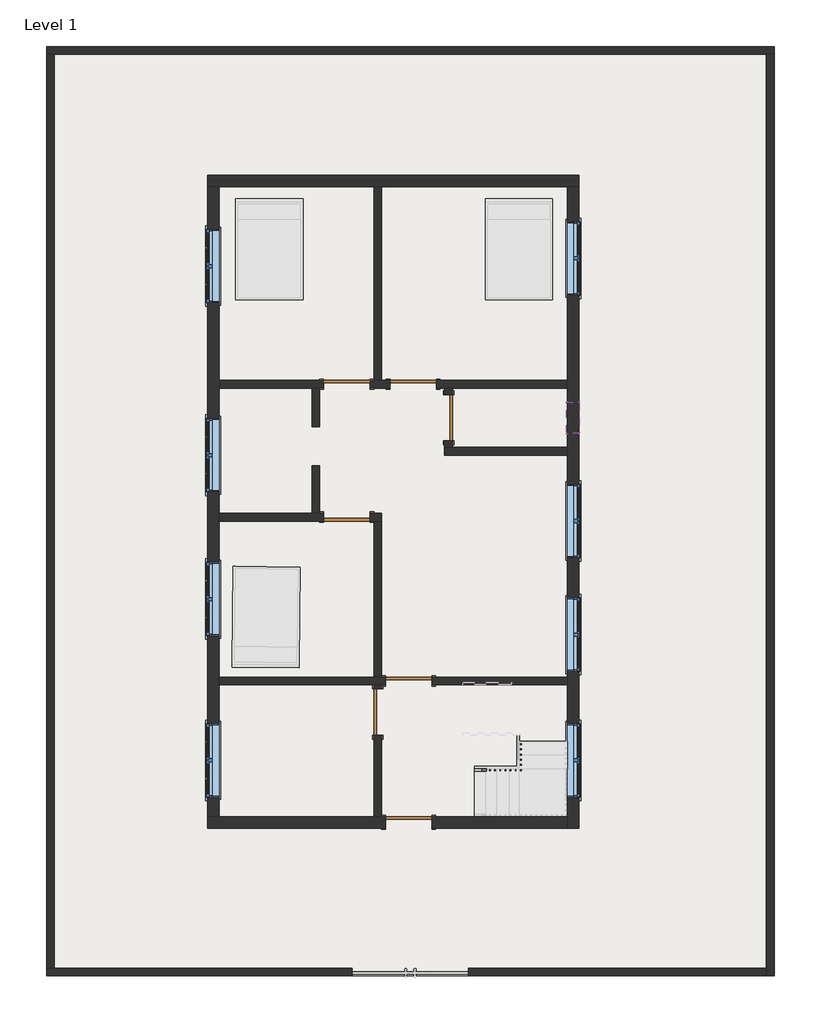
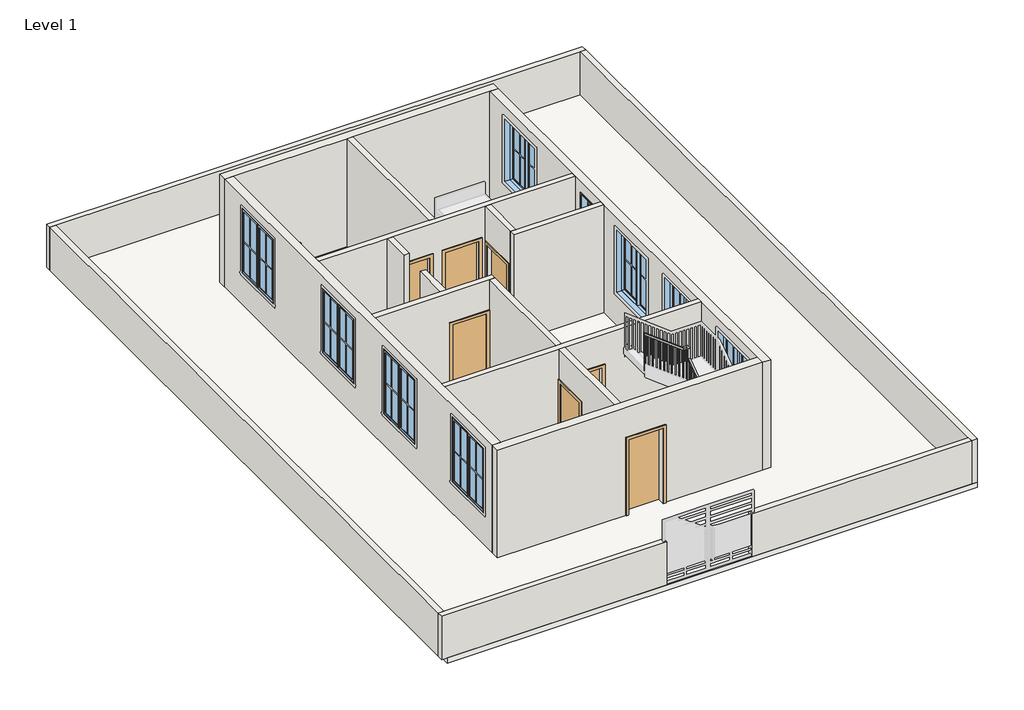
# One storey, part 1 of 2: 19 walls, 9 windows, 7 doors, 1 railing, 1 slab.
"""IFC4 building model written with IfcOpenShell, lengths in millimetres."""

from ifc_helpers import new_model, si_unit, frame, origin, origin_with_axes, place, context, project, spatial, polyline, outline, extrude, faceted_brep, transform, mapped, element, save
from components import door_2b0b55a0, door_686f89d2, door_16372e1c, door_a90ba1ad, window_9ac97e1a, window_f2d8fef0

model = new_model("IFC4")

# Units and contexts
model_context = context("Model", 3, world=origin())
ifc_project = project(units=[si_unit("LENGTHUNIT", "METRE", prefix="MILLI")], contexts=[model_context])

# Site, building, storey
site = spatial("IfcSite", under=ifc_project)
building = spatial("IfcBuilding", under=site)
storey = spatial("IfcBuildingStorey", under=building, Name="Level 1", Elevation=0.0)

# Doors
placement = place(None, origin())
door_shape = door_2b0b55a0(model_context)
element("IfcDoor", 1, ObjectType="Single-Flush : 36\" x 80\"", at=placement, inside=storey, context=model_context, shape_type="MappedRepresentation", body=[
    mapped(door_shape, transform((-163.235885, 1707.4649429, 0.0), x_axis=(0.0, 1.0, 0.0), y_axis=(-1.0, 0.0, 0.0), z_axis=(0.0, 0.0, 1.0))),
])
door_2_shape = door_686f89d2(model_context)
element("IfcDoor", 2, ObjectType="Single-Flush : 36\" x 84\"", at=placement, inside=storey, context=model_context, shape_type="MappedRepresentation", body=[
    mapped(door_2_shape, transform((-861.735885, 2367.8649429, 0.0), x_axis=(-1.0, 0.0, 0.0), y_axis=(0.0, -1.0, 0.0), z_axis=(0.0, 0.0, 1.0))),
])
element("IfcDoor", 3, ObjectType="Single-Flush : 36\" x 84\"", at=placement, inside=storey, context=model_context, shape_type="MappedRepresentation", body=[
    mapped(door_2_shape, transform((-2169.835885, -248.3350571, 0.0), x_axis=(1.0, 0.0, 0.0), y_axis=(0.0, 1.0, 0.0), z_axis=(0.0, 0.0, 1.0))),
])
element("IfcDoor", 4, ObjectType="Single-Flush : 36\" x 84\"", at=placement, inside=storey, context=model_context, shape_type="MappedRepresentation", body=[
    mapped(door_2_shape, transform((-950.635885, -3474.1350571, 0.0), x_axis=(-1.0, 0.0, 0.0), y_axis=(0.0, -1.0, 0.0), z_axis=(0.0, 0.0, 1.0))),
])
door_3_shape = door_16372e1c(model_context)
element("IfcDoor", 5, ObjectType="Single-Flush : 36\" x 84\"", at=placement, inside=storey, context=model_context, shape_type="MappedRepresentation", body=[
    mapped(door_3_shape, transform((-2169.835885, 2367.8649429, 0.0), x_axis=(1.0, 0.0, 0.0), y_axis=(0.0, 1.0, 0.0), z_axis=(0.0, 0.0, 1.0))),
])
element("IfcDoor", 6, ObjectType="Single-Flush : 36\" x 84\"", at=placement, inside=storey, context=model_context, shape_type="MappedRepresentation", body=[
    mapped(door_3_shape, transform((-1560.235885, -4083.7350571, 0.0), x_axis=(0.0, 1.0, 0.0), y_axis=(-1.0, 0.0, 0.0), z_axis=(0.0, 0.0, 1.0))),
])
door_4_shape = door_a90ba1ad(model_context)
element("IfcDoor", 7, ObjectType="Single-Flush : 36\" x 84\"", at=placement, inside=storey, context=model_context, shape_type="MappedRepresentation", body=[
    mapped(door_4_shape, transform((-950.635885, -6255.4350571, 0.0), x_axis=(-1.0, 0.0, 0.0), y_axis=(0.0, -1.0, 0.0), z_axis=(0.0, 0.0, 1.0))),
])

# Railing
element("IfcRailing", 8, ObjectType="Handrail - Rectangular", at=placement, inside=storey, context=model_context, shape_type="SolidModel", body=[
    faceted_brep([(344.764115, -5201.3350571, 1083.7333333), (344.764115, -5201.3350571, 1019.8686436), (344.764115, -5252.1350571, 1019.8686436), (344.764115, -5252.1350571, 1083.7333333), (1157.564115, -5201.3350571, 1703.0095238), (1208.364115, -5201.3350571, 1677.849596), (1208.364115, -5252.1350571, 1677.849596), (1157.564115, -5252.1350571, 1703.0095238), (1157.564115, -5201.3350571, 1984.8285714), (1208.364115, -5201.3350571, 1934.0285714), (1208.364115, -5252.1350571, 1934.0285714), (1157.564115, -5252.1350571, 1984.8285714), (1233.764115, -5201.3350571, 1984.8285714), (1233.764115, -5201.3350571, 1934.0285714), (1284.564115, -5252.1350571, 1934.0285714), (1284.564115, -5252.1350571, 1984.8285714), (1233.764115, -5125.1350571, 1984.8285714), (1233.764115, -5108.8554323, 1934.0285714), (1284.564115, -5108.8554323, 1934.0285714), (1284.564115, -5125.1350571, 1984.8285714), (1233.764115, -4566.3350571, 2383.9714286), (1233.764115, -4515.5350571, 2357.8288395), (1284.564115, -4515.5350571, 2357.8288395), (1284.564115, -4566.3350571, 2383.9714286), (1233.764115, -4566.3350571, 2665.4606061), (1233.764115, -4515.5350571, 2614.6606061), (1284.564115, -4515.5350571, 2614.6606061), (1284.564115, -4566.3350571, 2665.4606061), (1233.764115, -4490.1350571, 2665.4606061), (1233.764115, -4490.1350571, 2614.6606061), (1284.564115, -4439.3350571, 2614.6606061), (1284.564115, -4439.3350571, 2665.4606061), (1157.564115, -4490.1350571, 2665.4606061), (1140.4943334, -4490.1350571, 2614.6606061), (1140.4943334, -4439.3350571, 2614.6606061), (1157.564115, -4439.3350571, 2665.4606061), (116.164115, -4490.1350571, 3454.4), (116.164115, -4439.3350571, 3454.4), (116.164115, -4439.3350571, 3390.6683472), (116.164115, -4490.1350571, 3390.6683472)], [[[0, 1, 2, 3]], [[1, 0, 4, 5]], [[2, 1, 5, 6]], [[3, 2, 6, 7]], [[0, 3, 7, 4]], [[5, 4, 8, 9]], [[6, 5, 9, 10]], [[7, 6, 10, 11]], [[4, 7, 11, 8]], [[9, 8, 12, 13]], [[10, 9, 13, 14]], [[11, 10, 14, 15]], [[8, 11, 15, 12]], [[13, 12, 16, 17]], [[14, 13, 17, 18]], [[15, 14, 18, 19]], [[12, 15, 19, 16]], [[17, 16, 20, 21]], [[18, 17, 21, 22]], [[19, 18, 22, 23]], [[16, 19, 23, 20]], [[21, 20, 24, 25]], [[22, 21, 25, 26]], [[23, 22, 26, 27]], [[20, 23, 27, 24]], [[25, 24, 28, 29]], [[26, 25, 29, 30]], [[27, 26, 30, 31]], [[24, 27, 31, 28]], [[29, 28, 32, 33]], [[30, 29, 33, 34]], [[31, 30, 34, 35]], [[28, 31, 35, 32]], [[36, 37, 38, 39]], [[33, 32, 36, 39]], [[34, 33, 39, 38]], [[35, 34, 38, 37]], [[32, 35, 37, 36]]]),
    extrude(outline(polyline([(3378.6418321, 132.039115), (2370.6666667, 132.039115), (2370.6666667, 151.089115), (3364.2100139, 151.089115), (3378.6418321, 132.039115)])), frame((0.0, -4474.2600571, 0.0), z_axis=(0.0, 1.0, 0.0), x_axis=(0.0, 0.0, 1.0)), (0.0, 0.0, 1.0), 19.05),
    extrude(outline(polyline([(3301.6721351, 233.639115), (2370.6666667, 233.639115), (2370.6666667, 252.689115), (3287.2403169, 252.689115), (3301.6721351, 233.639115)])), frame((0.0, -4474.2600571, 0.0), z_axis=(0.0, 1.0, 0.0), x_axis=(0.0, 0.0, 1.0)), (0.0, 0.0, 1.0), 19.05),
    extrude(outline(polyline([(3224.7024382, 335.239115), (2370.6666667, 335.239115), (2370.6666667, 354.289115), (3210.27062, 354.289115), (3224.7024382, 335.239115)])), frame((0.0, -4474.2600571, 0.0), z_axis=(0.0, 1.0, 0.0), x_axis=(0.0, 0.0, 1.0)), (0.0, 0.0, 1.0), 19.05),
    extrude(outline(polyline([(3147.7327412, 436.839115), (2201.3333333, 436.839115), (2201.3333333, 455.889115), (3133.300923, 455.889115), (3147.7327412, 436.839115)])), frame((0.0, -4474.2600571, 0.0), z_axis=(0.0, 1.0, 0.0), x_axis=(0.0, 0.0, 1.0)), (0.0, 0.0, 1.0), 19.05),
    extrude(outline(polyline([(3070.7630442, 538.439115), (2201.3333333, 538.439115), (2201.3333333, 557.489115), (3056.331226, 557.489115), (3070.7630442, 538.439115)])), frame((0.0, -4474.2600571, 0.0), z_axis=(0.0, 1.0, 0.0), x_axis=(0.0, 0.0, 1.0)), (0.0, 0.0, 1.0), 19.05),
    extrude(outline(polyline([(2993.7933472, 640.039115), (2032.0, 640.039115), (2032.0, 659.089115), (2979.3615291, 659.089115), (2993.7933472, 640.039115)])), frame((0.0, -4474.2600571, 0.0), z_axis=(0.0, 1.0, 0.0), x_axis=(0.0, 0.0, 1.0)), (0.0, 0.0, 1.0), 19.05),
    extrude(outline(polyline([(2916.8236503, 741.639115), (2032.0, 741.639115), (2032.0, 760.689115), (2902.3918321, 760.689115), (2916.8236503, 741.639115)])), frame((0.0, -4474.2600571, 0.0), z_axis=(0.0, 1.0, 0.0), x_axis=(0.0, 0.0, 1.0)), (0.0, 0.0, 1.0), 19.05),
    extrude(outline(polyline([(2839.8539533, 843.239115), (1862.6666667, 843.239115), (1862.6666667, 862.289115), (2825.4221351, 862.289115), (2839.8539533, 843.239115)])), frame((0.0, -4474.2600571, 0.0), z_axis=(0.0, 1.0, 0.0), x_axis=(0.0, 0.0, 1.0)), (0.0, 0.0, 1.0), 19.05),
    extrude(outline(polyline([(2762.8842563, 944.839115), (1862.6666667, 944.839115), (1862.6666667, 963.889115), (2748.4524382, 963.889115), (2762.8842563, 944.839115)])), frame((0.0, -4474.2600571, 0.0), z_axis=(0.0, 1.0, 0.0), x_axis=(0.0, 0.0, 1.0)), (0.0, 0.0, 1.0), 19.05),
    extrude(outline(polyline([(2685.9145594, 1046.439115), (1693.3333333, 1046.439115), (1693.3333333, 1065.489115), (2671.4827412, 1065.489115), (2685.9145594, 1046.439115)])), frame((0.0, -4474.2600571, 0.0), z_axis=(0.0, 1.0, 0.0), x_axis=(0.0, 0.0, 1.0)), (0.0, 0.0, 1.0), 19.05),
    extrude(outline(polyline([(2608.9448624, 1148.039115), (1693.3333333, 1148.039115), (1693.3333333, 1167.089115), (2594.5130442, 1167.089115), (2608.9448624, 1148.039115)])), frame((0.0, -4474.2600571, 0.0), z_axis=(0.0, 1.0, 0.0), x_axis=(0.0, 0.0, 1.0)), (0.0, 0.0, 1.0), 19.05),
    extrude(outline(polyline([(1249.639115, -4525.0600571), (1249.639115, -4506.0100571), (1268.689115, -4506.0100571), (1268.689115, -4525.0600571), (1249.639115, -4525.0600571)])), frame((0.0, 0.0, 1354.6666667), z_axis=(0.0, 0.0, 1.0), x_axis=(1.0, 0.0, 0.0)), (0.0, 0.0, 1.0), 1259.9939394),
    extrude(outline(polyline([(-4607.6100571, 2292.0609823), (-4607.6100571, 1354.6666667), (-4626.6600571, 1354.6666667), (-4626.6600571, 2278.4538395), (-4607.6100571, 2292.0609823)])), frame((1249.639115, 0.0, 0.0), z_axis=(1.0, 0.0, 0.0), x_axis=(0.0, 1.0, 0.0)), (0.0, 0.0, 1.0), 19.05),
    extrude(outline(polyline([(-4709.2100571, 2219.4895538), (-4709.2100571, 1185.3333333), (-4728.2600571, 1185.3333333), (-4728.2600571, 2205.8824109), (-4709.2100571, 2219.4895538)])), frame((1249.639115, 0.0, 0.0), z_axis=(1.0, 0.0, 0.0), x_axis=(0.0, 1.0, 0.0)), (0.0, 0.0, 1.0), 19.05),
    extrude(outline(polyline([(-4810.8100571, 2146.9181252), (-4810.8100571, 1185.3333333), (-4829.8600571, 1185.3333333), (-4829.8600571, 2133.3109823), (-4810.8100571, 2146.9181252)])), frame((1249.639115, 0.0, 0.0), z_axis=(1.0, 0.0, 0.0), x_axis=(0.0, 1.0, 0.0)), (0.0, 0.0, 1.0), 19.05),
    extrude(outline(polyline([(-4912.4100571, 2074.3466966), (-4912.4100571, 1185.3333333), (-4931.4600571, 1185.3333333), (-4931.4600571, 2060.7395538), (-4912.4100571, 2074.3466966)])), frame((1249.639115, 0.0, 0.0), z_axis=(1.0, 0.0, 0.0), x_axis=(0.0, 1.0, 0.0)), (0.0, 0.0, 1.0), 19.05),
    extrude(outline(polyline([(-5014.0100571, 2001.7752681), (-5014.0100571, 1016.0), (-5033.0600571, 1016.0), (-5033.0600571, 1988.1681252), (-5014.0100571, 2001.7752681)])), frame((1249.639115, 0.0, 0.0), z_axis=(1.0, 0.0, 0.0), x_axis=(0.0, 1.0, 0.0)), (0.0, 0.0, 1.0), 19.05),
    extrude(outline(polyline([(-5115.6100571, 1929.2038395), (-5115.6100571, 1016.0), (-5134.6600571, 1016.0), (-5134.6600571, 1915.5966966), (-5115.6100571, 1929.2038395)])), frame((1249.639115, 0.0, 0.0), z_axis=(1.0, 0.0, 0.0), x_axis=(0.0, 1.0, 0.0)), (0.0, 0.0, 1.0), 19.05),
    extrude(outline(polyline([(1631.8876912, 1148.039115), (677.3333333, 1148.039115), (677.3333333, 1167.089115), (1646.4019769, 1167.089115), (1631.8876912, 1148.039115)])), frame((0.0, -5236.2600571, 0.0), z_axis=(0.0, 1.0, 0.0), x_axis=(0.0, 0.0, 1.0)), (0.0, 0.0, 1.0), 19.05),
    extrude(outline(polyline([(1554.4781674, 1046.439115), (677.3333333, 1046.439115), (677.3333333, 1065.489115), (1568.9924531, 1065.489115), (1554.4781674, 1046.439115)])), frame((0.0, -5236.2600571, 0.0), z_axis=(0.0, 1.0, 0.0), x_axis=(0.0, 0.0, 1.0)), (0.0, 0.0, 1.0), 19.05),
    extrude(outline(polyline([(1477.0686436, 944.839115), (508.0, 944.839115), (508.0, 963.889115), (1491.5829293, 963.889115), (1477.0686436, 944.839115)])), frame((0.0, -5236.2600571, 0.0), z_axis=(0.0, 1.0, 0.0), x_axis=(0.0, 0.0, 1.0)), (0.0, 0.0, 1.0), 19.05),
    extrude(outline(polyline([(1399.6591198, 843.239115), (508.0, 843.239115), (508.0, 862.289115), (1414.1734055, 862.289115), (1399.6591198, 843.239115)])), frame((0.0, -5236.2600571, 0.0), z_axis=(0.0, 1.0, 0.0), x_axis=(0.0, 0.0, 1.0)), (0.0, 0.0, 1.0), 19.05),
    extrude(outline(polyline([(1322.249596, 741.639115), (338.6666667, 741.639115), (338.6666667, 760.689115), (1336.7638817, 760.689115), (1322.249596, 741.639115)])), frame((0.0, -5236.2600571, 0.0), z_axis=(0.0, 1.0, 0.0), x_axis=(0.0, 0.0, 1.0)), (0.0, 0.0, 1.0), 19.05),
    extrude(outline(polyline([(1244.8400722, 640.039115), (338.6666667, 640.039115), (338.6666667, 659.089115), (1259.3543579, 659.089115), (1244.8400722, 640.039115)])), frame((0.0, -5236.2600571, 0.0), z_axis=(0.0, 1.0, 0.0), x_axis=(0.0, 0.0, 1.0)), (0.0, 0.0, 1.0), 19.05),
    extrude(outline(polyline([(1167.4305484, 538.439115), (169.3333333, 538.439115), (169.3333333, 557.489115), (1181.9448341, 557.489115), (1167.4305484, 538.439115)])), frame((0.0, -5236.2600571, 0.0), z_axis=(0.0, 1.0, 0.0), x_axis=(0.0, 0.0, 1.0)), (0.0, 0.0, 1.0), 19.05),
    extrude(outline(polyline([(1090.0210246, 436.839115), (169.3333333, 436.839115), (169.3333333, 455.889115), (1104.5353103, 455.889115), (1090.0210246, 436.839115)])), frame((0.0, -5236.2600571, 0.0), z_axis=(0.0, 1.0, 0.0), x_axis=(0.0, 0.0, 1.0)), (0.0, 0.0, 1.0), 19.05),
    extrude(outline(polyline([(1249.639115, -4474.2600571), (1249.639115, -4455.2100571), (1268.689115, -4455.2100571), (1268.689115, -4474.2600571), (1249.639115, -4474.2600571)])), frame((0.0, 0.0, 1524.0), z_axis=(0.0, 0.0, 1.0), x_axis=(1.0, 0.0, 0.0)), (0.0, 0.0, 1.0), 1090.6606061),
    extrude(outline(polyline([(1249.639115, -5217.2100571), (1268.689115, -5217.2100571), (1268.689115, -5236.2600571), (1249.639115, -5236.2600571), (1249.639115, -5217.2100571)])), frame((0.0, 0.0, 846.6666667), z_axis=(0.0, 0.0, 1.0), x_axis=(1.0, 0.0, 0.0)), (0.0, 0.0, 1.0), 1087.3619048),
    extrude(outline(polyline([(3390.6683472, 116.164115), (2370.6666667, 116.164115), (2370.6666667, 135.214115), (3376.2365291, 135.214115), (3390.6683472, 116.164115)])), frame((0.0, -4474.2600571, 0.0), z_axis=(0.0, 1.0, 0.0), x_axis=(0.0, 0.0, 1.0)), (0.0, 0.0, 1.0), 19.05),
    extrude(outline(polyline([(1019.8686436, 344.764115), (169.3333333, 344.764115), (169.3333333, 363.814115), (1034.3829293, 363.814115), (1019.8686436, 344.764115)])), frame((0.0, -5236.2600571, 0.0), z_axis=(0.0, 1.0, 0.0), x_axis=(0.0, 0.0, 1.0)), (0.0, 0.0, 1.0), 19.05),
])

# Slab
element("IfcSlab", 9, ObjectType="FLOOR 6\"", at=placement, inside=storey, context=model_context, shape_type="SweptSolid", body=[
    extrude(outline(polyline([(6245.0981003, 9012.3928288), (6245.0981003, -9275.6071712), (-7928.1018997, -9275.6071712), (-7928.1018997, 9012.3928288), (6245.0981003, 9012.3928288)])), frame((0.0, 0.0, -152.4), z_axis=(0.0, 0.0, 1.0), x_axis=(1.0, 0.0, 0.0)), (0.0, 0.0, 1.0), 152.4),
])

# Walls
element("IfcWall", 10, ObjectType="CMD 6\"", at=placement, inside=storey, context=model_context, shape_type="Brep", body=[
    faceted_brep([(-8080.5018997, 8859.9928288, 0.0), (-7928.1018997, 8859.9928288, 0.0), (6092.6981003, 8859.9928288, 0.0), (6245.0981003, 8859.9928288, 0.0), (6245.0981003, 8859.9928288, 1219.2), (6092.6981003, 8859.9928288, 1219.2), (-7928.1018997, 8859.9928288, 1219.2), (-8080.5018997, 8859.9928288, 1219.2), (-8080.5018997, 9012.3928288, 0.0), (-8080.5018997, 9012.3928288, 1219.2), (6245.0981003, 9012.3928288, 1219.2), (6245.0981003, 9012.3928288, 0.0)], [[[0, 1, 2, 3, 4, 5, 6, 7]], [[8, 9, 10, 11]], [[3, 2, 1, 0, 8, 11]], [[7, 6, 5, 4, 10, 9]], [[4, 3, 11, 10]], [[0, 7, 9, 8]]]),
])
element("IfcWall", 11, ObjectType="CMD 6\"", at=placement, inside=storey, context=model_context, shape_type="Brep", body=[
    faceted_brep([(6092.6981003, 8859.9928288, 0.0), (6092.6981003, -9123.2071712, 0.0), (6092.6981003, -9275.6071712, 0.0), (6092.6981003, -9275.6071712, 1219.2), (6092.6981003, -9123.2071712, 1219.2), (6092.6981003, 8859.9928288, 1219.2), (6245.0981003, 8859.9928288, 0.0), (6245.0981003, 8859.9928288, 1219.2), (6245.0981003, -9275.6071712, 1219.2), (6245.0981003, -9275.6071712, 0.0)], [[[0, 1, 2, 3, 4, 5]], [[6, 7, 8, 9]], [[2, 1, 0, 6, 9]], [[5, 4, 3, 8, 7]], [[0, 5, 7, 6]], [[3, 2, 9, 8]]]),
])
element("IfcWall", 12, ObjectType="CMD 6\"", at=placement, inside=storey, context=model_context, shape_type="SweptSolid", body=[
    extrude(outline(polyline([(225.2981003, -9123.2071712), (6092.6981003, -9123.2071712), (6092.6981003, -9275.6071712), (225.2981003, -9275.6071712), (225.2981003, -9123.2071712)])), origin_with_axes(), (0.0, 0.0, 1.0), 1219.2),
])
element("IfcWall", 13, ObjectType="CMD 6\"", at=placement, inside=storey, context=model_context, shape_type="SweptSolid", body=[
    extrude(outline(polyline([(-7928.1018997, 8859.9928288), (-7928.1018997, -9123.2071712), (-8080.5018997, -9123.2071712), (-8080.5018997, 8859.9928288), (-7928.1018997, 8859.9928288)])), origin_with_axes(), (0.0, 0.0, 1.0), 1219.2),
])
element("IfcWall", 14, ObjectType="CMD 6\"", at=placement, inside=storey, context=model_context, shape_type="Brep", body=[
    faceted_brep([(-2060.7018997, -9123.2071712, 0.0), (-7928.1018997, -9123.2071712, 0.0), (-8080.5018997, -9123.2071712, 0.0), (-8080.5018997, -9123.2071712, 1219.2), (-7928.1018997, -9123.2071712, 1219.2), (-2060.7018997, -9123.2071712, 1219.2), (-2060.7018997, -9275.6071712, 0.0), (-2060.7018997, -9275.6071712, 1219.2), (-8080.5018997, -9275.6071712, 1219.2), (-8080.5018997, -9275.6071712, 0.0)], [[[0, 1, 2, 3, 4, 5]], [[6, 7, 8, 9]], [[2, 1, 0, 6, 9]], [[5, 4, 3, 8, 7]], [[0, 5, 7, 6]], [[3, 2, 9, 8]]]),
])
element("IfcWall", 15, ObjectType="WALL 6\"", at=placement, inside=storey, context=model_context, shape_type="SweptSolid", body=[
    extrude(outline(polyline([(-1636.435885, 2444.0649429), (-1636.435885, 6254.0649429), (-1484.035885, 6254.0649429), (-1484.035885, 2444.0649429), (-1636.435885, 2444.0649429)])), origin_with_axes(), (0.0, 0.0, 1.0), 3048.0),
])
element("IfcWall", 16, ObjectType="WALL 6\"", at=placement, inside=storey, context=model_context, shape_type="Brep", body=[
    faceted_brep([(-1318.935885, 2444.0649429, 0.0), (-1484.035885, 2444.0649429, 0.0), (-1636.435885, 2444.0649429, 0.0), (-1712.635885, 2444.0649429, 0.0), (-1712.635885, 2444.0649429, 2133.6), (-2627.035885, 2444.0649429, 2133.6), (-2627.035885, 2444.0649429, 0.0), (-4684.435885, 2444.0649429, 0.0), (-4684.435885, 2444.0649429, 3048.0), (-1636.435885, 2444.0649429, 3048.0), (-1484.035885, 2444.0649429, 3048.0), (2173.564115, 2444.0649429, 3048.0), (2173.564115, 2444.0649429, 0.0), (-404.535885, 2444.0649429, 0.0), (-404.535885, 2444.0649429, 2133.6), (-1318.935885, 2444.0649429, 2133.6), (-1712.635885, 2291.6649429, 2133.6), (-1712.635885, 2291.6649429, 0.0), (-1318.935885, 2291.6649429, 0.0), (-1318.935885, 2291.6649429, 2133.6), (-404.535885, 2291.6649429, 2133.6), (-404.535885, 2291.6649429, 0.0), (-239.435885, 2291.6649429, 0.0), (-87.035885, 2291.6649429, 0.0), (2173.564115, 2291.6649429, 0.0), (2173.564115, 2291.6649429, 3048.0), (-87.035885, 2291.6649429, 3048.0), (-239.435885, 2291.6649429, 3048.0), (-2703.235885, 2291.6649429, 3048.0), (-2855.635885, 2291.6649429, 3048.0), (-4684.435885, 2291.6649429, 3048.0), (-4684.435885, 2291.6649429, 0.0), (-2855.635885, 2291.6649429, 0.0), (-2703.235885, 2291.6649429, 0.0), (-2627.035885, 2291.6649429, 0.0), (-2627.035885, 2291.6649429, 2133.6)], [[[0, 1, 2, 3, 4, 5, 6, 7, 8, 9, 10, 11, 12, 13, 14, 15]], [[16, 17, 18, 19, 20, 21, 22, 23, 24, 25, 26, 27, 28, 29, 30, 31, 32, 33, 34, 35]], [[13, 12, 24, 23, 22, 21]], [[18, 17, 3, 2, 1, 0]], [[34, 33, 32, 31, 7, 6]], [[12, 11, 25, 24]], [[8, 7, 31, 30]], [[19, 18, 0, 15]], [[20, 19, 15, 14]], [[21, 20, 14, 13]], [[4, 3, 17, 16]], [[5, 4, 16, 35]], [[6, 5, 35, 34]], [[11, 10, 9, 8, 30, 29, 28, 27, 26, 25]]]),
])
element("IfcWall", 17, ObjectType="WALL 6\"", at=placement, inside=storey, context=model_context, shape_type="SweptSolid", body=[
    extrude(outline(polyline([(-2855.635885, 1529.6649429), (-2855.635885, 2291.6649429), (-2703.235885, 2291.6649429), (-2703.235885, 1529.6649429), (-2855.635885, 1529.6649429)])), origin_with_axes(), (0.0, 0.0, 1.0), 3048.0),
])
element("IfcWall", 18, ObjectType="WALL 6\"", at=placement, inside=storey, context=model_context, shape_type="Brep", body=[
    faceted_brep([(-1712.635885, -324.5350571, 2133.6), (-1712.635885, -324.5350571, 0.0), (-1636.435885, -324.5350571, 0.0), (-1484.035885, -324.5350571, 0.0), (-1484.035885, -324.5350571, 3048.0), (-1636.435885, -324.5350571, 3048.0), (-4684.435885, -324.5350571, 3048.0), (-4684.435885, -324.5350571, 0.0), (-2627.035885, -324.5350571, 0.0), (-2627.035885, -324.5350571, 2133.6), (-1484.035885, -172.1350571, 0.0), (-1712.635885, -172.1350571, 0.0), (-1712.635885, -172.1350571, 2133.6), (-2627.035885, -172.1350571, 2133.6), (-2627.035885, -172.1350571, 0.0), (-2703.235885, -172.1350571, 0.0), (-2855.635885, -172.1350571, 0.0), (-4684.435885, -172.1350571, 0.0), (-4684.435885, -172.1350571, 3048.0), (-2855.635885, -172.1350571, 3048.0), (-2703.235885, -172.1350571, 3048.0), (-1484.035885, -172.1350571, 3048.0)], [[[0, 1, 2, 3, 4, 5, 6, 7, 8, 9]], [[10, 11, 12, 13, 14, 15, 16, 17, 18, 19, 20, 21]], [[8, 7, 17, 16, 15, 14]], [[3, 2, 1, 11, 10]], [[7, 6, 18, 17]], [[4, 3, 10, 21]], [[12, 11, 1, 0]], [[13, 12, 0, 9]], [[14, 13, 9, 8]], [[6, 5, 4, 21, 20, 19, 18]]]),
])
element("IfcWall", 19, ObjectType="WALL 6\"", at=placement, inside=storey, context=model_context, shape_type="SweptSolid", body=[
    extrude(outline(polyline([(-1636.435885, -3397.9350571), (-1636.435885, -324.5350571), (-1484.035885, -324.5350571), (-1484.035885, -3397.9350571), (-1636.435885, -3397.9350571)])), origin_with_axes(), (0.0, 0.0, 1.0), 3048.0),
])
element("IfcWall", 20, ObjectType="WALL 6\"", at=placement, inside=storey, context=model_context, shape_type="Brep", body=[
    faceted_brep([(-4684.435885, -3550.3350571, 0.0), (-1636.435885, -3550.3350571, 0.0), (-1484.035885, -3550.3350571, 0.0), (-1407.835885, -3550.3350571, 0.0), (-1407.835885, -3550.3350571, 2133.6), (-493.435885, -3550.3350571, 2133.6), (-493.435885, -3550.3350571, 0.0), (2173.564115, -3550.3350571, 0.0), (2173.564115, -3550.3350571, 3048.0), (-1484.035885, -3550.3350571, 3048.0), (-1636.435885, -3550.3350571, 3048.0), (-4684.435885, -3550.3350571, 3048.0), (-1407.835885, -3397.9350571, 2133.6), (-1407.835885, -3397.9350571, 0.0), (-1484.035885, -3397.9350571, 0.0), (-1636.435885, -3397.9350571, 0.0), (-4684.435885, -3397.9350571, 0.0), (-4684.435885, -3397.9350571, 3048.0), (-1636.435885, -3397.9350571, 3048.0), (-1484.035885, -3397.9350571, 3048.0), (2173.564115, -3397.9350571, 3048.0), (2173.564115, -3397.9350571, 0.0), (-493.435885, -3397.9350571, 0.0), (-493.435885, -3397.9350571, 2133.6)], [[[0, 1, 2, 3, 4, 5, 6, 7, 8, 9, 10, 11]], [[12, 13, 14, 15, 16, 17, 18, 19, 20, 21, 22, 23]], [[22, 21, 7, 6]], [[16, 15, 14, 13, 3, 2, 1, 0]], [[8, 7, 21, 20]], [[0, 11, 17, 16]], [[4, 3, 13, 12]], [[5, 4, 12, 23]], [[6, 5, 23, 22]], [[11, 10, 9, 8, 20, 19, 18, 17]]]),
])
element("IfcWall", 21, ObjectType="WALL 6\"", at=placement, inside=storey, context=model_context, shape_type="SweptSolid", body=[
    extrude(outline(polyline([(-3550.3350571, 0.0), (-3626.5350571, 0.0), (-3626.5350571, 2133.6), (-4540.9350571, 2133.6), (-4540.9350571, 0.0), (-6141.1350571, 0.0), (-6141.1350571, 3048.0), (-3550.3350571, 3048.0), (-3550.3350571, 0.0)])), frame((-1636.435885, 0.0, 0.0), z_axis=(1.0, 0.0, 0.0), x_axis=(0.0, 1.0, 0.0)), (0.0, 0.0, 1.0), 152.4),
])
element("IfcWall", 22, ObjectType="WALL 6\"", at=placement, inside=storey, context=model_context, shape_type="Brep", body=[
    faceted_brep([(2173.564115, 1123.2649429, 0.0), (-87.035885, 1123.2649429, 0.0), (-239.435885, 1123.2649429, 0.0), (-239.435885, 1123.2649429, 3048.0), (-87.035885, 1123.2649429, 3048.0), (2173.564115, 1123.2649429, 3048.0), (2173.564115, 970.8649429, 0.0), (2173.564115, 970.8649429, 3048.0), (-239.435885, 970.8649429, 3048.0), (-239.435885, 970.8649429, 0.0)], [[[0, 1, 2, 3, 4, 5]], [[6, 7, 8, 9]], [[2, 1, 0, 6, 9]], [[0, 5, 7, 6]], [[3, 2, 9, 8]], [[5, 4, 3, 8, 7]]]),
])
element("IfcWall", 23, ObjectType="WALL 6\"", at=placement, inside=storey, context=model_context, shape_type="SweptSolid", body=[
    extrude(outline(polyline([(2291.6649429, 0.0), (2164.6649429, 0.0), (2164.6649429, 2032.0), (1250.2649429, 2032.0), (1250.2649429, 0.0), (1123.2649429, 0.0), (1123.2649429, 3048.0), (2291.6649429, 3048.0), (2291.6649429, 0.0)])), frame((-239.435885, 0.0, 0.0), z_axis=(1.0, 0.0, 0.0), x_axis=(0.0, 1.0, 0.0)), (0.0, 0.0, 1.0), 152.4),
])
element("IfcWall", 24, ObjectType="WALL 6\"", at=placement, inside=storey, context=model_context, shape_type="SweptSolid", body=[
    extrude(outline(polyline([(-2855.635885, -172.1350571), (-2855.635885, 767.6649429), (-2703.235885, 767.6649429), (-2703.235885, -172.1350571), (-2855.635885, -172.1350571)])), origin_with_axes(), (0.0, 0.0, 1.0), 3048.0),
])
element("IfcWall", 25, ObjectType="WALL 9\"", at=placement, inside=storey, context=model_context, shape_type="Brep", body=[
    faceted_brep([(-4913.035885, 6254.0649429, 0.0), (-4684.435885, 6254.0649429, 0.0), (-1636.435885, 6254.0649429, 0.0), (-1484.035885, 6254.0649429, 0.0), (2173.564115, 6254.0649429, 0.0), (2402.164115, 6254.0649429, 0.0), (2402.164115, 6254.0649429, 3048.0), (2173.564115, 6254.0649429, 3048.0), (-1484.035885, 6254.0649429, 3048.0), (-1636.435885, 6254.0649429, 3048.0), (-4684.435885, 6254.0649429, 3048.0), (-4913.035885, 6254.0649429, 3048.0), (-4913.035885, 6482.6649429, 0.0), (-4913.035885, 6482.6649429, 3048.0), (2402.164115, 6482.6649429, 3048.0), (2402.164115, 6482.6649429, 0.0)], [[[0, 1, 2, 3, 4, 5, 6, 7, 8, 9, 10, 11]], [[12, 13, 14, 15]], [[5, 4, 3, 2, 1, 0, 12, 15]], [[6, 5, 15, 14]], [[0, 11, 13, 12]], [[11, 10, 9, 8, 7, 6, 14, 13]]]),
])
element("IfcWall", 26, ObjectType="WALL 9\"", at=placement, inside=storey, context=model_context, shape_type="Brep", body=[
    faceted_brep([(2173.564115, 6254.0649429, 0.0), (2173.564115, 2444.0649429, 0.0), (2173.564115, 2291.6649429, 0.0), (2173.564115, 1123.2649429, 0.0), (2173.564115, 970.8649429, 0.0), (2173.564115, -3397.9350571, 0.0), (2173.564115, -3550.3350571, 0.0), (2173.564115, -6141.1350571, 0.0), (2173.564115, -6369.7350571, 0.0), (2173.564115, -6369.7350571, 3048.0), (2173.564115, -6141.1350571, 3048.0), (2173.564115, -3550.3350571, 3048.0), (2173.564115, -3397.9350571, 3048.0), (2173.564115, 970.8649429, 3048.0), (2173.564115, 1123.2649429, 3048.0), (2173.564115, 2291.6649429, 3048.0), (2173.564115, 2444.0649429, 3048.0), (2173.564115, 6254.0649429, 3048.0), (2173.564115, -5760.1350571, 2743.2), (2173.564115, -5760.1350571, 914.4), (2173.564115, -4312.3350571, 914.4), (2173.564115, -4312.3350571, 2743.2), (2173.564115, -3283.6350571, 2743.2), (2173.564115, -3283.6350571, 914.4), (2173.564115, -1835.8350571, 914.4), (2173.564115, -1835.8350571, 2743.2), (2173.564115, -1048.4350571, 2743.2), (2173.564115, -1048.4350571, 914.4), (2173.564115, 399.3649429, 914.4), (2173.564115, 399.3649429, 2743.2), (2173.564115, 4120.4649429, 2743.2), (2173.564115, 4120.4649429, 914.4), (2173.564115, 5568.2649429, 914.4), (2173.564115, 5568.2649429, 2743.2), (2173.564115, 2012.2649429, 2743.2), (2173.564115, 1402.6649429, 2743.2), (2173.564115, 1402.6649429, 2133.6), (2173.564115, 2012.2649429, 2133.6), (2402.164115, 6254.0649429, 0.0), (2402.164115, 6254.0649429, 3048.0), (2402.164115, -6369.7350571, 3048.0), (2402.164115, -6369.7350571, 0.0), (2402.164115, -5760.1350571, 2743.2), (2402.164115, -4312.3350571, 2743.2), (2402.164115, -4312.3350571, 914.4), (2402.164115, -5760.1350571, 914.4), (2402.164115, -3283.6350571, 2743.2), (2402.164115, -1835.8350571, 2743.2), (2402.164115, -1835.8350571, 914.4), (2402.164115, -3283.6350571, 914.4), (2402.164115, -1048.4350571, 2743.2), (2402.164115, 399.3649429, 2743.2), (2402.164115, 399.3649429, 914.4), (2402.164115, -1048.4350571, 914.4), (2402.164115, 4120.4649429, 2743.2), (2402.164115, 5568.2649429, 2743.2), (2402.164115, 5568.2649429, 914.4), (2402.164115, 4120.4649429, 914.4), (2402.164115, 2012.2649429, 2743.2), (2402.164115, 2012.2649429, 2133.6), (2402.164115, 1402.6649429, 2133.6), (2402.164115, 1402.6649429, 2743.2)], [[[0, 1, 2, 3, 4, 5, 6, 7, 8, 9, 10, 11, 12, 13, 14, 15, 16, 17], [18, 19, 20, 21], [22, 23, 24, 25], [26, 27, 28, 29], [30, 31, 32, 33], [34, 35, 36, 37]], [[38, 39, 40, 41], [42, 43, 44, 45], [46, 47, 48, 49], [50, 51, 52, 53], [54, 55, 56, 57], [58, 59, 60, 61]], [[8, 7, 6, 5, 4, 3, 2, 1, 0, 38, 41]], [[0, 17, 39, 38]], [[9, 8, 41, 40]], [[19, 18, 42, 45]], [[20, 19, 45, 44]], [[21, 20, 44, 43]], [[18, 21, 43, 42]], [[23, 22, 46, 49]], [[24, 23, 49, 48]], [[25, 24, 48, 47]], [[22, 25, 47, 46]], [[27, 26, 50, 53]], [[28, 27, 53, 52]], [[29, 28, 52, 51]], [[26, 29, 51, 50]], [[31, 30, 54, 57]], [[32, 31, 57, 56]], [[33, 32, 56, 55]], [[30, 33, 55, 54]], [[59, 58, 34, 37]], [[60, 59, 37, 36]], [[61, 60, 36, 35]], [[58, 61, 35, 34]], [[17, 16, 15, 14, 13, 12, 11, 10, 9, 40, 39]]]),
])
element("IfcWall", 27, ObjectType="WALL 9\"", at=placement, inside=storey, context=model_context, shape_type="Brep", body=[
    faceted_brep([(-1407.835885, -6141.1350571, 2133.6), (-1407.835885, -6141.1350571, 0.0), (-1484.035885, -6141.1350571, 0.0), (-1636.435885, -6141.1350571, 0.0), (-4684.435885, -6141.1350571, 0.0), (-4913.035885, -6141.1350571, 0.0), (-4913.035885, -6141.1350571, 3048.0), (-4684.435885, -6141.1350571, 3048.0), (-1636.435885, -6141.1350571, 3048.0), (-1484.035885, -6141.1350571, 3048.0), (2173.564115, -6141.1350571, 3048.0), (2173.564115, -6141.1350571, 0.0), (-493.435885, -6141.1350571, 0.0), (-493.435885, -6141.1350571, 2133.6), (-4913.035885, -6369.7350571, 0.0), (-1407.835885, -6369.7350571, 0.0), (-1407.835885, -6369.7350571, 2133.6), (-493.435885, -6369.7350571, 2133.6), (-493.435885, -6369.7350571, 0.0), (2173.564115, -6369.7350571, 0.0), (2173.564115, -6369.7350571, 3048.0), (-4913.035885, -6369.7350571, 3048.0)], [[[0, 1, 2, 3, 4, 5, 6, 7, 8, 9, 10, 11, 12, 13]], [[14, 15, 16, 17, 18, 19, 20, 21]], [[12, 11, 19, 18]], [[5, 4, 3, 2, 1, 15, 14]], [[11, 10, 20, 19]], [[6, 5, 14, 21]], [[16, 15, 1, 0]], [[17, 16, 0, 13]], [[18, 17, 13, 12]], [[10, 9, 8, 7, 6, 21, 20]]]),
])
element("IfcWall", 28, ObjectType="WALL 9\"", at=placement, inside=storey, context=model_context, shape_type="Brep", body=[
    faceted_brep([(-4684.435885, -6141.1350571, 0.0), (-4684.435885, -3550.3350571, 0.0), (-4684.435885, -3397.9350571, 0.0), (-4684.435885, -324.5350571, 0.0), (-4684.435885, -172.1350571, 0.0), (-4684.435885, 2291.6649429, 0.0), (-4684.435885, 2444.0649429, 0.0), (-4684.435885, 6254.0649429, 0.0), (-4684.435885, 6254.0649429, 3048.0), (-4684.435885, 2444.0649429, 3048.0), (-4684.435885, 2291.6649429, 3048.0), (-4684.435885, -172.1350571, 3048.0), (-4684.435885, -324.5350571, 3048.0), (-4684.435885, -3397.9350571, 3048.0), (-4684.435885, -3550.3350571, 3048.0), (-4684.435885, -6141.1350571, 3048.0), (-4684.435885, -4312.3350571, 2743.2), (-4684.435885, -4312.3350571, 914.4), (-4684.435885, -5760.1350571, 914.4), (-4684.435885, -5760.1350571, 2743.2), (-4684.435885, -1137.3350571, 2743.2), (-4684.435885, -1137.3350571, 914.4), (-4684.435885, -2585.1350571, 914.4), (-4684.435885, -2585.1350571, 2743.2), (-4684.435885, 1694.7649429, 2743.2), (-4684.435885, 1694.7649429, 914.4), (-4684.435885, 246.9649429, 914.4), (-4684.435885, 246.9649429, 2743.2), (-4684.435885, 5415.8649429, 2743.2), (-4684.435885, 5415.8649429, 914.4), (-4684.435885, 3968.0649429, 914.4), (-4684.435885, 3968.0649429, 2743.2), (-4913.035885, -6141.1350571, 0.0), (-4913.035885, -6141.1350571, 3048.0), (-4913.035885, 6254.0649429, 3048.0), (-4913.035885, 6254.0649429, 0.0), (-4913.035885, -4312.3350571, 2743.2), (-4913.035885, -5760.1350571, 2743.2), (-4913.035885, -5760.1350571, 914.4), (-4913.035885, -4312.3350571, 914.4), (-4913.035885, -1137.3350571, 2743.2), (-4913.035885, -2585.1350571, 2743.2), (-4913.035885, -2585.1350571, 914.4), (-4913.035885, -1137.3350571, 914.4), (-4913.035885, 1694.7649429, 2743.2), (-4913.035885, 246.9649429, 2743.2), (-4913.035885, 246.9649429, 914.4), (-4913.035885, 1694.7649429, 914.4), (-4913.035885, 5415.8649429, 2743.2), (-4913.035885, 3968.0649429, 2743.2), (-4913.035885, 3968.0649429, 914.4), (-4913.035885, 5415.8649429, 914.4)], [[[0, 1, 2, 3, 4, 5, 6, 7, 8, 9, 10, 11, 12, 13, 14, 15], [16, 17, 18, 19], [20, 21, 22, 23], [24, 25, 26, 27], [28, 29, 30, 31]], [[32, 33, 34, 35], [36, 37, 38, 39], [40, 41, 42, 43], [44, 45, 46, 47], [48, 49, 50, 51]], [[7, 6, 5, 4, 3, 2, 1, 0, 32, 35]], [[8, 7, 35, 34]], [[0, 15, 33, 32]], [[17, 16, 36, 39]], [[18, 17, 39, 38]], [[19, 18, 38, 37]], [[16, 19, 37, 36]], [[21, 20, 40, 43]], [[22, 21, 43, 42]], [[23, 22, 42, 41]], [[20, 23, 41, 40]], [[25, 24, 44, 47]], [[26, 25, 47, 46]], [[27, 26, 46, 45]], [[24, 27, 45, 44]], [[29, 28, 48, 51]], [[30, 29, 51, 50]], [[31, 30, 50, 49]], [[28, 31, 49, 48]], [[15, 14, 13, 12, 11, 10, 9, 8, 34, 33]]]),
])

# Windows
window_shape = window_9ac97e1a(model_context)
element("IfcWindow", 29, ObjectType="Window-Casement-Double : 57\" x 72\"", at=placement, inside=storey, context=model_context, shape_type="MappedRepresentation", body=[
    mapped(window_shape, transform((-4798.735885, -5036.2350571, 0.0), x_axis=(0.0, 1.0, 0.0), y_axis=(-1.0, 0.0, 0.0), z_axis=(0.0, 0.0, 1.0))),
])
element("IfcWindow", 30, ObjectType="Window-Casement-Double : 57\" x 72\"", at=placement, inside=storey, context=model_context, shape_type="MappedRepresentation", body=[
    mapped(window_shape, transform((2287.864115, -5036.2350571, 0.0), x_axis=(0.0, -1.0, 0.0), y_axis=(1.0, 0.0, 0.0), z_axis=(0.0, 0.0, 1.0))),
])
element("IfcWindow", 31, ObjectType="Window-Casement-Double : 57\" x 72\"", at=placement, inside=storey, context=model_context, shape_type="MappedRepresentation", body=[
    mapped(window_shape, transform((2287.864115, -2559.7350571, 0.0), x_axis=(0.0, -1.0, 0.0), y_axis=(1.0, 0.0, 0.0), z_axis=(0.0, 0.0, 1.0))),
])
element("IfcWindow", 32, ObjectType="Window-Casement-Double : 57\" x 72\"", at=placement, inside=storey, context=model_context, shape_type="MappedRepresentation", body=[
    mapped(window_shape, transform((2287.864115, -324.5350571, 0.0), x_axis=(0.0, -1.0, 0.0), y_axis=(1.0, 0.0, 0.0), z_axis=(0.0, 0.0, 1.0))),
])
element("IfcWindow", 33, ObjectType="Window-Casement-Double : 57\" x 72\"", at=placement, inside=storey, context=model_context, shape_type="MappedRepresentation", body=[
    mapped(window_shape, transform((-4798.735885, -1861.2350571, 0.0), x_axis=(0.0, 1.0, 0.0), y_axis=(-1.0, 0.0, 0.0), z_axis=(0.0, 0.0, 1.0))),
])
element("IfcWindow", 34, ObjectType="Window-Casement-Double : 57\" x 72\"", at=placement, inside=storey, context=model_context, shape_type="MappedRepresentation", body=[
    mapped(window_shape, transform((-4798.735885, 970.8649429, 0.0), x_axis=(0.0, 1.0, 0.0), y_axis=(-1.0, 0.0, 0.0), z_axis=(0.0, 0.0, 1.0))),
])
element("IfcWindow", 35, ObjectType="Window-Casement-Double : 57\" x 72\"", at=placement, inside=storey, context=model_context, shape_type="MappedRepresentation", body=[
    mapped(window_shape, transform((-4798.735885, 4691.9649429, 0.0), x_axis=(0.0, 1.0, 0.0), y_axis=(-1.0, 0.0, 0.0), z_axis=(0.0, 0.0, 1.0))),
])
element("IfcWindow", 36, ObjectType="Window-Casement-Double : 57\" x 72\"", at=placement, inside=storey, context=model_context, shape_type="MappedRepresentation", body=[
    mapped(window_shape, transform((2287.864115, 4844.3649429, 0.0), x_axis=(0.0, -1.0, 0.0), y_axis=(1.0, 0.0, 0.0), z_axis=(0.0, 0.0, 1.0))),
])
window_2_shape = window_f2d8fef0(model_context)
element("IfcWindow", 37, ObjectType="Window-Louvers : 24\" x 24\"", at=placement, inside=storey, context=model_context, shape_type="MappedRepresentation", body=[
    mapped(window_2_shape, transform((2294.214115, 1707.4649429, 1219.2), x_axis=(0.0, -1.0, 0.0), y_axis=(1.0, 0.0, 0.0), z_axis=(0.0, 0.0, 1.0))),
])

save(model, "model.ifc")

# Revit data of these elements
# Type "Single-Flush : 36\" x 80\""
#   Type Mark = "6"
#   Construction Type Id = "MDOOR"
#   Assembly Code = "C1020"
#   Analytic Construction = "Metal"
#   Thickness = 0' - 2"
#   Heat Transfer Coefficient (U) = 0.651978 BTU/(h·ft²·°F)
#   Height = 6' - 8"
#   Trim Projection Ext = 0' - 1"
#   Trim Projection Int = 0' - 1"
#   Trim Width = 0' - 3"
#   Width = 3' - 0"
#   Define Thermal Properties by = 1
#   Define Thermal Properties by = 1
#   Door Material = Door - Panel
#   Frame Material = Door - Frame
#   Visual Light Transmittance = 0
#   Solar Heat Gain Coefficient = 0
#   Function = (empty or 0)
#   Wall Closure = (empty or 0)
# Type "Single-Flush : 36\" x 84\""
#   Type Mark = "1"
#   Construction Type Id = "MDOOR"
#   Assembly Code = "C1020"
#   Analytic Construction = "Metal"
#   Thickness = 0' - 2"
#   Heat Transfer Coefficient (U) = 0.651978 BTU/(h·ft²·°F)
#   Height = 7' - 0"
#   Trim Projection Ext = 0' - 1"
#   Trim Projection Int = 0' - 1"
#   Trim Width = 0' - 3"
#   Width = 3' - 0"
#   Define Thermal Properties by = 1
#   Define Thermal Properties by = 1
#   Door Material = Door - Panel
#   Frame Material = Door - Frame
#   Visual Light Transmittance = 0
#   Solar Heat Gain Coefficient = 0
#   Function = (empty or 0)
#   Wall Closure = (empty or 0)
# Type "Handrail - Rectangular"
#   Assembly Code = "C2010400"
#   built-in parameter 1008612 = 0.0416667 (stored number, unit not read)
#   built-in parameter 1008611 = 0.0416667 (stored number, unit not read)
#   built-in parameter 1008609 = 0.333333 (stored number, unit not read)
#   built-in parameter 1008604 = 0.166667 (stored number, unit not read)
#   built-in parameter 1008603 = 0.166667 (stored number, unit not read)
#   Railing Height = 3' - 0"
#   built-in parameter 1008630 = 2
#   built-in parameter 1008610 = 2
#   built-in parameter 1008618 = Baluster - Square : 3/4"
# Type "FLOOR 6\""
#   Assembly Code = "B1010"
#   Function = 0
#   Layers, outside or top first: 0' - 6" no material (function 1)
# Type "CMD 6\""
#   Assembly Code = "B2010"
#   Layers, outside or top first: 0' - 6" no material (function 1)
# Type "WALL 6\""
#   Assembly Code = "B2010"
#   Layers, outside or top first: 0' - 6" no material (function 1)
# Type "WALL 9\""
#   Assembly Code = "B2010"
#   Layers, outside or top first: 0' - 9" no material (function 1)
# Type "Window-Casement-Double : 57\" x 72\""
#   Type Mark = "17"
#   Fire Rating = "0.5h"
#   Assembly Code = "B2020100"
#   Analytic Construction = "Double glazing - domestic"
#   Frame Extension [instance default] = 0' - 0 1/4"
#   Window Inset [instance default] = 0' - 0"
#   Wall Thickness [instance default] = 0' - 6"
#   Interior Wall Closure [instance default] = 0' - 2 1/4"
#   Half Width = 2' - 4 1/2"
#   Visual Light Transmittance = 0.81
#   Thermal Resistance (R) = 1.8146 (h·ft²·°F)/BTU
#   Solar Heat Gain Coefficient = 0.76
#   Rough Width = 4' - 9 1/2"
#   Rough Height = 6' - 0 1/2"
#   Height = 6' - 0"
#   Heat Transfer Coefficient (U) = 0.5511 BTU/(h·ft²·°F)
#   Exterior Wall Closure [instance default] = 0' - 1 1/4"
#   Extension Jamb [instance default] = 0' - 2 1/4"
#   Default Sill Height = 3' - 0"
#   Width = 4' - 9"
#   Define Thermal Properties by = 0
#   Muntin Visibility = yes
#   Interior Trim Visibility [instance default] = yes
#   Exterior Trim Visibility [instance default] = yes
#   Extension Jamb Visibility [instance default] = yes
#   Interior Trim Material = Wood - Stained
#   Muntin Pattern = Muntin Pattern_2x2 : Muntin Pattern_2x2
#   Interior Trim = Trim-Window-Interior-Flat : Picture Frame
#   Interior Frame Material = Wood - Stained
#   Glass Panel Material = Glass
#   Exterior Trim Material = Clad - White
#   Exterior Trim = Trim-Window-Exterior-Flat : with Sill
#   Exterior Frame Material = Clad - White
#   Wall Closure = (empty or 0)
# Type "Window-Louvers : 24\" x 24\""
#   Type Mark = "18"
#   Construction Type Id = "GSP4R"
#   Assembly Code = "B20"
#   Analytic Construction = "1/8 in Pilkington single glazing"
#   Visual Light Transmittance = 0.9
#   Thermal Resistance (R) = 1.53941 (h·ft²·°F)/BTU
#   Solar Heat Gain Coefficient = 0.78
#   Max Height = 1' - 11.74264"
#   Height = 2' - 0"
#   Heat Transfer Coefficient (U) = 0.6496 BTU/(h·ft²·°F)
#   Blade Width [instance default] = 1' - 10 1/2"
#   Blade Vertical Thickness = 0' - 0.35355"
#   Blade Thickness = 0' - 0 1/4"
#   Blade Spacing = 0' - 1 1/2"
#   Blade Height = 0' - 1.85355"
#   Blade Depth = 0' - 3"
#   Blade Angle = 45.00°
#   Default Sill Height = 3' - 0"
#   Trim Projection_Exterior = 0' - 0 1/2"
#   Trim Projection_Interior = 0' - 0 1/2"
#   Trim Width_Exterior = 0' - 1 1/2"
#   Trim Width_Interior = 0' - 1 1/2"
#   Width = 2' - 0"
#   Max Blade Count = 12
#   Define Thermal Properties by = 1
#   Blade Count = 12
#   Frame Material = Birch
#   Louver Material = Birch
#   Trim Exterior Material = Birch
#   Trim Interior Material = Birch
#   Wall Closure = (empty or 0)
# Element 1 (IfcDoor, "Single-Flush : 36\" x 80\"")
#   Phase Created = New Construction
#   Materials on its faces: "Door - Frame", "Door - Panel"
# Elements 2, 3, 4, 5, 6, 7 (IfcDoor, "Single-Flush : 36\" x 84\"")
#   Phase Created = New Construction
#   Materials on its faces: "Door - Frame", "Door - Panel"
# Element 8 (IfcRailing, "Handrail - Rectangular")
#   Phase Created = New Construction
# Element 9 (IfcSlab, "FLOOR 6\"")
#   Height Offset From Level = 0' - 0"
#   Phase Created = New Construction
#   Materials on its faces: "Default Floor", "Door - Panel"
# Elements 10, 11, 12, 13 (IfcWall, "CMD 6\"")
#   Top Offset = 0' - 0"
#   Base Offset = 0' - 0"
#   Unconnected Height = 4' - 0"
#   wall height = 4' - 0"
#   Phase Created = New Construction
#   Base Constraint = Level 1
#   Materials on its faces: "Default Wall", "Clad - White"
# Element 14 (IfcWall, "CMD 6\"")
#   Top Offset = 0' - 0"
#   Base Offset = 0' - 0"
#   Unconnected Height = 4' - 0"
#   wall height = 4' - 0"
#   Phase Created = New Construction
#   Base Constraint = Level 1
#   Materials on its faces: "Clad - White", "Default Wall"
# Elements 15, 16, 17, 18, 19, 20, 21, 22, 23, 24 (IfcWall, "WALL 6\"")
#   Top Offset = 0' - 0"
#   Base Offset = 0' - 0"
#   Unconnected Height = 10' - 0"
#   wall height = 10' - 0"
#   Phase Created = New Construction
#   Base Constraint = Level 1
#   Materials on its faces: "Default Wall"
# Elements 25, 26, 27, 28 (IfcWall, "WALL 9\"")
#   Top Offset = 0' - 0"
#   Base Offset = 0' - 0"
#   Unconnected Height = 10' - 0"
#   wall height = 10' - 0"
#   Phase Created = New Construction
#   Base Constraint = Level 1
#   Materials on its faces: "Default Wall", "Cherry"
# Element 29 (IfcWindow, "Window-Casement-Double : 57\" x 72\"")
#   Mark = "1"
#   Window Inset = 0' - 0"
#   Interior Wall Closure = 0' - 2 1/4"
#   Frame Extension = 0' - 0 1/4"
#   Exterior Wall Closure = 0' - 1 1/4"
#   Interior Trim Visibility = yes
#   Exterior Trim Visibility = yes
#   Phase Created = New Construction
#   Materials on its faces: "Wood - Stained", "Glass", "Clad - White"
# Element 30 (IfcWindow, "Window-Casement-Double : 57\" x 72\"")
#   Mark = "2"
#   Window Inset = 0' - 0"
#   Interior Wall Closure = 0' - 2 1/4"
#   Frame Extension = 0' - 0 1/4"
#   Exterior Wall Closure = 0' - 1 1/4"
#   Interior Trim Visibility = yes
#   Exterior Trim Visibility = yes
#   Phase Created = New Construction
#   Materials on its faces: "Wood - Stained", "Glass", "Clad - White"
# Element 31 (IfcWindow, "Window-Casement-Double : 57\" x 72\"")
#   Mark = "3"
#   Window Inset = 0' - 0"
#   Interior Wall Closure = 0' - 2 1/4"
#   Frame Extension = 0' - 0 1/4"
#   Exterior Wall Closure = 0' - 1 1/4"
#   Interior Trim Visibility = yes
#   Exterior Trim Visibility = yes
#   Phase Created = New Construction
#   Materials on its faces: "Wood - Stained", "Glass", "Clad - White"
# Element 32 (IfcWindow, "Window-Casement-Double : 57\" x 72\"")
#   Mark = "4"
#   Window Inset = 0' - 0"
#   Interior Wall Closure = 0' - 2 1/4"
#   Frame Extension = 0' - 0 1/4"
#   Exterior Wall Closure = 0' - 1 1/4"
#   Interior Trim Visibility = yes
#   Exterior Trim Visibility = yes
#   Phase Created = New Construction
#   Materials on its faces: "Wood - Stained", "Glass", "Clad - White"
# Element 33 (IfcWindow, "Window-Casement-Double : 57\" x 72\"")
#   Mark = "5"
#   Window Inset = 0' - 0"
#   Interior Wall Closure = 0' - 2 1/4"
#   Frame Extension = 0' - 0 1/4"
#   Exterior Wall Closure = 0' - 1 1/4"
#   Interior Trim Visibility = yes
#   Exterior Trim Visibility = yes
#   Phase Created = New Construction
#   Materials on its faces: "Wood - Stained", "Glass", "Clad - White"
# Element 34 (IfcWindow, "Window-Casement-Double : 57\" x 72\"")
#   Mark = "6"
#   Window Inset = 0' - 0"
#   Interior Wall Closure = 0' - 2 1/4"
#   Frame Extension = 0' - 0 1/4"
#   Exterior Wall Closure = 0' - 1 1/4"
#   Interior Trim Visibility = yes
#   Exterior Trim Visibility = yes
#   Phase Created = New Construction
#   Materials on its faces: "Wood - Stained", "Glass", "Clad - White"
# Element 35 (IfcWindow, "Window-Casement-Double : 57\" x 72\"")
#   Mark = "7"
#   Window Inset = 0' - 0"
#   Interior Wall Closure = 0' - 2 1/4"
#   Frame Extension = 0' - 0 1/4"
#   Exterior Wall Closure = 0' - 1 1/4"
#   Interior Trim Visibility = yes
#   Exterior Trim Visibility = yes
#   Phase Created = New Construction
#   Materials on its faces: "Wood - Stained", "Glass", "Clad - White"
# Element 36 (IfcWindow, "Window-Casement-Double : 57\" x 72\"")
#   Mark = "8"
#   Window Inset = 0' - 0"
#   Interior Wall Closure = 0' - 2 1/4"
#   Frame Extension = 0' - 0 1/4"
#   Exterior Wall Closure = 0' - 1 1/4"
#   Interior Trim Visibility = yes
#   Exterior Trim Visibility = yes
#   Phase Created = New Construction
#   Materials on its faces: "Wood - Stained", "Glass", "Clad - White"
# Element 37 (IfcWindow, "Window-Louvers : 24\" x 24\"")
#   Mark = "9"
#   Blade Width = 1' - 10 1/2"
#   Phase Created = New Construction
#   Materials on its faces: "Birch"
# Materials
#   "Door - Panel": class "Wood", colour RGB 210 159 95, transparency 0, Cost = 0
#   "Door - Frame": colour RGB 118 70 51, transparency 0, Cost = 0
#   "Wood - Stained": class "Wood", colour RGB 224 178 126, transparency 0, Cost = 0
#   "Glass": class "Glass", colour RGB 0 128 192, transparency 0.75, Description = "Soda Lime Glass", Cost = 0
#   "Clad - White": class "Wood", colour RGB 242 242 238, transparency 0, Cost = 0
#   "Birch": class "Wood", colour RGB 224 178 126, transparency 0, Description = "Betula Alleghaniensis", Cost = 0
#   "Default Floor": colour RGB 128 128 128, transparency 0, Cost = 0
#   "Default Wall": colour RGB 128 128 128, transparency 0, Cost = 0
#   "Cherry": class "Wood", colour RGB 226 177 128, transparency 0, Description = "Prunus Serotina", Cost = 0
